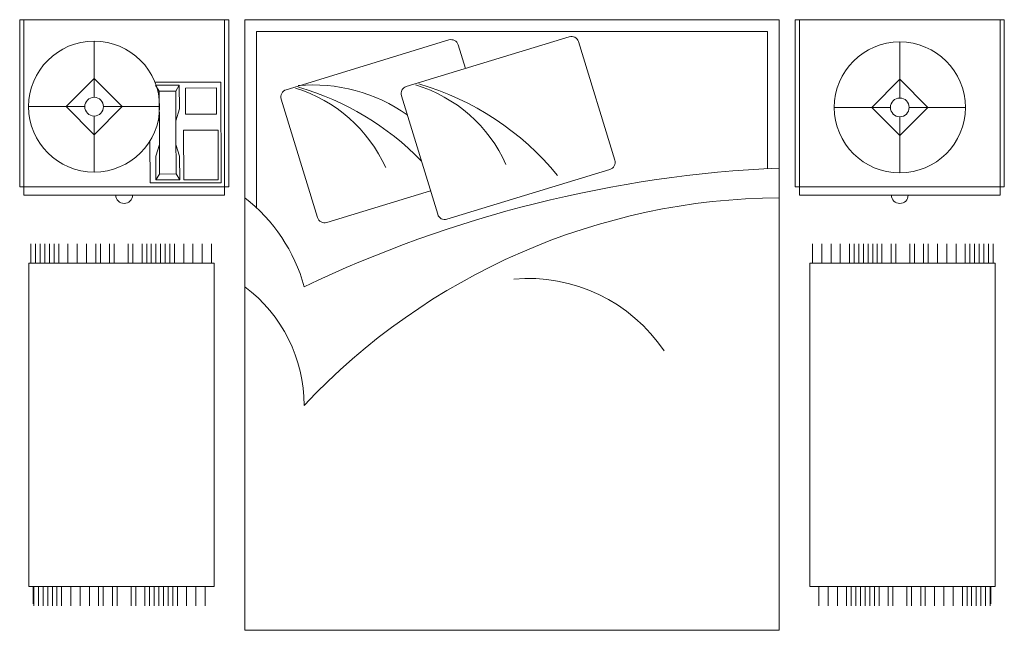
# Model space of a CAD drawing. Units: inches. Extents: x 1994 to 3075, y 3517 to 3950.
# Tile 30 of 58: x 1994.4586 to 1994.5883, y 3553.6956 to 3553.7761. Entities that reach past the tile are written whole.
import ezdxf

# ---------------------------------------------------------------- set-up
doc = ezdxf.new("R2010")
doc.units = ezdxf.units.IN
doc.layers.add('A-FURN-REFR', color=8, linetype='Continuous', lineweight=13)

msp = doc.modelspace()

# ---------------------------------------------------------------- linework, layer by layer
at = {"layer": 'A-FURN-REFR'}
for p, q in [((1994.45855170359, 3553.754079419354), (1994.45855170359, 3553.776112109586)), ((1994.45855170359, 3553.776112109586), (1994.486092566381, 3553.776112109586)), ((1994.459102520846, 3553.752977784842), (1994.459102520846, 3553.776112109586)), ((1994.485541749125, 3553.776112109586), (1994.485541749125, 3553.752977784842)), ((1994.486092566381, 3553.776112109586), (1994.486092566381, 3553.754079419354)), ((1994.488211515722, 3553.776112109586), (1994.488211515722, 3553.752634222582)), ((1994.558645176735, 3553.776112109586), (1994.488211515722, 3553.776112109586)), ((1994.558645176735, 3553.756547203749), (1994.558645176735, 3553.776112109586)), ((1994.560764126075, 3553.776112109586), (1994.560764126075, 3553.754077215864)), ((1994.588307743228, 3553.776112109586), (1994.560764126075, 3553.776112109586)), ((1994.561314998418, 3553.776112109586), (1994.561314998418, 3553.752975471179)), ((1994.587756870884, 3553.752975471179), (1994.587756870884, 3553.776112109586)), ((1994.588307743228, 3553.754077215864), (1994.588307743228, 3553.776112109586)), ((1994.468361056407, 3553.773278802821), (1994.468361056407, 3553.765875817668)), ((1994.515123148426, 3553.773437261622), (1994.493655292272, 3553.766868059838)), ((1994.530971129343, 3553.773869308913), (1994.509503273189, 3553.767300107129)), ((1994.516344913196, 3553.772788026205), (1994.517294663113, 3553.769684286165)), ((1994.532192894112, 3553.773220073496), (1994.536976663113, 3553.757586931427)), ((1994.574535934651, 3553.773181469956), (1994.574535934651, 3553.765777744431)), ((1994.464659560746, 3553.764641987016), (1994.468361056407, 3553.768343480208)), ((1994.468361056407, 3553.768343480208), (1994.472062548366, 3553.764641987016)), ((1994.485054603369, 3553.767890645299), (1994.476376887084, 3553.76785773335)), ((1994.485104968809, 3553.754611060531), (1994.485054603369, 3553.767890645299)), ((1994.574535934651, 3553.768245653762), (1994.570834072506, 3553.764543790383)), ((1994.578237800498, 3553.764543790383), (1994.574535934651, 3553.768245653762)), ((1994.476463412208, 3553.767467479873), (1994.479588020389, 3553.767479330565)), ((1994.476935066108, 3553.766688105432), (1994.476463412208, 3553.767467479873)), ((1994.476935066108, 3553.766688105432), (1994.479122291835, 3553.766696400916)), ((1994.476955804819, 3553.761220041116), (1994.476935066108, 3553.766688105432)), ((1994.479588020389, 3553.767479330565), (1994.479122291835, 3553.766696400916)), ((1994.479143030545, 3553.7612283366), (1994.479122291835, 3553.766696400916)), ((1994.479588020389, 3553.767479330565), (1994.47959987108, 3553.764354722384)), ((1994.493006056854, 3553.765646295068), (1994.497789825855, 3553.750013152999)), ((1994.508854037771, 3553.766078342358), (1994.513637806771, 3553.75044520029)), ((1994.467127225754, 3553.764641987016), (1994.459724238134, 3553.764641987016)), ((1994.468361056407, 3553.760940495056), (1994.464659560746, 3553.764641987016)), ((1994.472062548366, 3553.764641987016), (1994.468361056407, 3553.760940495056)), ((1994.46959488706, 3553.764641987016), (1994.476997870978, 3553.764641987016)), ((1994.47959987108, 3553.764354722384), (1994.479137105199, 3553.762790640691)), ((1994.573301980603, 3553.764543790383), (1994.565898256312, 3553.764543790383)), ((1994.570834072506, 3553.764543790383), (1994.574535934651, 3553.760841928237)), ((1994.574535934651, 3553.760841928237), (1994.578237800498, 3553.764543790383)), ((1994.5757698887, 3553.764543790383), (1994.583173616692, 3553.764543790383)), ((1994.468361056407, 3553.76340815698), (1994.468361056407, 3553.756005173678)), ((1994.476856918961, 3553.763087996861), (1994.476949879473, 3553.762782345206)), ((1994.574535934651, 3553.763309836951), (1994.574535934651, 3553.755906113277)), ((1994.476955804819, 3553.761220041116), (1994.47697654353, 3553.755751976799)), ((1994.479143030545, 3553.7612283366), (1994.479163769256, 3553.755760272284)), ((1994.475710172916, 3553.760104911694), (1994.475731144267, 3553.754575508455)), ((1994.476498964283, 3553.758093655331), (1994.476961730165, 3553.759657737025)), ((1994.479623572464, 3553.758105506023), (1994.479148955892, 3553.759666032509)), ((1994.476510814975, 3553.75496904715), (1994.476498964283, 3553.758093655331)), ((1994.479635423156, 3553.754980897842), (1994.479623572464, 3553.758105506023)), ((1994.536327427695, 3553.756365166657), (1994.514859571541, 3553.749795964872)), ((1994.558645176735, 3553.756547203749), (1994.558645176735, 3553.695576880486)), ((1994.475731144267, 3553.754575508455), (1994.485104968809, 3553.754611060531)), ((1994.47697654353, 3553.755751976799), (1994.476510814975, 3553.75496904715)), ((1994.476510814975, 3553.75496904715), (1994.479635423156, 3553.754980897842)), ((1994.47697654353, 3553.755751976799), (1994.479163769256, 3553.755760272284)), ((1994.479635423156, 3553.754980897842), (1994.479163769256, 3553.755760272284)), ((1994.486092566381, 3553.754079419354), (1994.45855170359, 3553.754079419354)), ((1994.512688056854, 3553.75354894033), (1994.499011590624, 3553.749363917582)), ((1994.560764126075, 3553.754077215864), (1994.588307743228, 3553.754077215864)), ((1994.485541749125, 3553.752977784842), (1994.459102520846, 3553.752977784842)), ((1994.488211515722, 3553.752634222582), (1994.488211515722, 3553.695576880486)), ((1994.561314998418, 3553.752975471179), (1994.587756870884, 3553.752975471179)), ((1994.460028788472, 3553.746531228937, -0.0358017680513295), (1994.460028788472, 3553.743990908382, -0.0358017680513295)), ((1994.460639045881, 3553.746531228937, -0.0358017680513295), (1994.460639045881, 3553.743990908382, -0.0358017680513295)), ((1994.460639045881, 3553.746531228937, -0.0358017680513295), (1994.460639045881, 3553.743990908382, -0.0358017680513295)), ((1994.461249303291, 3553.746531228937, -0.0358017680513295), (1994.461249303291, 3553.743990908382, -0.0358017680513295)), ((1994.461859560701, 3553.746531228937, -0.0358017680513295), (1994.461859560701, 3553.743990908382, -0.0358017680513295)), ((1994.462469818111, 3553.746531228937, -0.0358017680513295), (1994.462469818111, 3553.743990908382, -0.0358017680513295)), ((1994.463080075522, 3553.746531228937, -0.0358017680513295), (1994.463080075522, 3553.743990908382, -0.0358017680513295)), ((1994.463690332931, 3553.746531228937, -0.0358017680513295), (1994.463690332931, 3553.743990908382, -0.0358017680513295)), ((1994.464910847751, 3553.746531228937, -0.0358017680513295), (1994.464910847751, 3553.743990908382, -0.0358017680513295)), ((1994.466131362571, 3553.746531228937, -0.0358017680513295), (1994.466131362571, 3553.743990908382, -0.0358017680513295)), ((1994.467351877391, 3553.746531228937, -0.0358017680513295), (1994.467351877391, 3553.743990908382, -0.0358017680513295)), ((1994.467351877391, 3553.746531228937, -0.0358017680513295), (1994.467351877391, 3553.743990908382, -0.0358017680513295)), ((1994.468572392211, 3553.746531228937, -0.0358017680513295), (1994.468572392211, 3553.743990908382, -0.0358017680513295)), ((1994.469182649621, 3553.746531228937, -0.0358017680513295), (1994.469182649621, 3553.743990908382, -0.0358017680513295)), ((1994.470403164441, 3553.746531228937, -0.0358017680513295), (1994.470403164441, 3553.743990908382, -0.0358017680513295)), ((1994.471013421851, 3553.746531228937, -0.0358017680513295), (1994.471013421851, 3553.743990908382, -0.0358017680513295)), ((1994.472844194081, 3553.746531228937, -0.0358017680513295), (1994.472844194081, 3553.743990908382, -0.0358017680513295)), ((1994.473454451491, 3553.746531228937, -0.0358017680513295), (1994.473454451491, 3553.743990908382, -0.0358017680513295)), ((1994.47467496631, 3553.746531228937, -0.0358017680513295), (1994.47467496631, 3553.743990908382, -0.0358017680513295)), ((1994.475285223721, 3553.746531228937, -0.0358017680513295), (1994.475285223721, 3553.743990908382, -0.0358017680513295)), ((1994.47589548113, 3553.746531228937, -0.0358017680513295), (1994.47589548113, 3553.743990908382, -0.0358017680513295)), ((1994.476505738541, 3553.746531228937, -0.0358017680513295), (1994.476505738541, 3553.743990908382, -0.0358017680513295)), ((1994.47711599595, 3553.746531228937, -0.0358017680513295), (1994.47711599595, 3553.743990908382, -0.0358017680513295)), ((1994.47772625336, 3553.746531228937, -0.0358017680513295), (1994.47772625336, 3553.743990908382, -0.0358017680513295)), ((1994.478336510771, 3553.746531228937, -0.0358017680513295), (1994.478336510771, 3553.743990908382, -0.0358017680513295)), ((1994.47894676818, 3553.746531228937, -0.0358017680513295), (1994.47894676818, 3553.743990908382, -0.0358017680513295)), ((1994.480167283, 3553.746531228937, -0.0358017680513295), (1994.480167283, 3553.743990908382, -0.0358017680513295)), ((1994.48138779782, 3553.746531228937, -0.0358017680513295), (1994.48138779782, 3553.743990908382, -0.0358017680513295)), ((1994.48260831264, 3553.746531228937, -0.0358017680513295), (1994.48260831264, 3553.743990908382, -0.0358017680513295)), ((1994.48382882746, 3553.746531228937, -0.0358017680513295), (1994.48382882746, 3553.743990908382, -0.0358017680513295)), ((1994.563027864996, 3553.746531228937, -0.0358017680513295), (1994.563027864996, 3553.743990908382, -0.0358017680513295)), ((1994.564248379816, 3553.746531228937, -0.0358017680513295), (1994.564248379816, 3553.743990908382, -0.0358017680513295)), ((1994.565468894636, 3553.746531228937, -0.0358017680513295), (1994.565468894636, 3553.743990908382, -0.0358017680513295)), ((1994.566689409456, 3553.746531228937, -0.0358017680513295), (1994.566689409456, 3553.743990908382, -0.0358017680513295)), ((1994.567909924276, 3553.746531228937, -0.0358017680513295), (1994.567909924276, 3553.743990908382, -0.0358017680513295)), ((1994.568520181686, 3553.746531228937, -0.0358017680513295), (1994.568520181686, 3553.743990908382, -0.0358017680513295)), ((1994.569130439096, 3553.746531228937, -0.0358017680513295), (1994.569130439096, 3553.743990908382, -0.0358017680513295)), ((1994.569740696505, 3553.746531228937, -0.0358017680513295), (1994.569740696505, 3553.743990908382, -0.0358017680513295)), ((1994.570350953916, 3553.746531228937, -0.0358017680513295), (1994.570350953916, 3553.743990908382, -0.0358017680513295)), ((1994.570961211326, 3553.746531228937, -0.0358017680513295), (1994.570961211326, 3553.743990908382, -0.0358017680513295)), ((1994.571571468735, 3553.746531228937, -0.0358017680513295), (1994.571571468735, 3553.743990908382, -0.0358017680513295)), ((1994.572181726146, 3553.746531228937, -0.0358017680513295), (1994.572181726146, 3553.743990908382, -0.0358017680513295)), ((1994.573402240965, 3553.746531228937, -0.0358017680513295), (1994.573402240965, 3553.743990908382, -0.0358017680513295)), ((1994.574012498375, 3553.746531228937, -0.0358017680513295), (1994.574012498375, 3553.743990908382, -0.0358017680513295)), ((1994.575843270605, 3553.746531228937, -0.0358017680513295), (1994.575843270605, 3553.743990908382, -0.0358017680513295)), ((1994.576453528015, 3553.746531228937, -0.0358017680513295), (1994.576453528015, 3553.743990908382, -0.0358017680513295)), ((1994.577674042835, 3553.746531228937, -0.0358017680513295), (1994.577674042835, 3553.743990908382, -0.0358017680513295)), ((1994.578284300245, 3553.746531228937, -0.0358017680513295), (1994.578284300245, 3553.743990908382, -0.0358017680513295)), ((1994.579504815065, 3553.746531228937, -0.0358017680513295), (1994.579504815065, 3553.743990908382, -0.0358017680513295)), ((1994.579504815065, 3553.746531228937, -0.0358017680513295), (1994.579504815065, 3553.743990908382, -0.0358017680513295)), ((1994.580725329885, 3553.746531228937, -0.0358017680513295), (1994.580725329885, 3553.743990908382, -0.0358017680513295)), ((1994.581945844705, 3553.746531228937, -0.0358017680513295), (1994.581945844705, 3553.743990908382, -0.0358017680513295)), ((1994.583166359525, 3553.746531228937, -0.0358017680513295), (1994.583166359525, 3553.743990908382, -0.0358017680513295)), ((1994.583776616935, 3553.746531228937, -0.0358017680513295), (1994.583776616935, 3553.743990908382, -0.0358017680513295)), ((1994.584386874345, 3553.746531228937, -0.0358017680513295), (1994.584386874345, 3553.743990908382, -0.0358017680513295)), ((1994.584997131755, 3553.746531228937, -0.0358017680513295), (1994.584997131755, 3553.743990908382, -0.0358017680513295)), ((1994.585607389165, 3553.746531228937, -0.0358017680513295), (1994.585607389165, 3553.743990908382, -0.0358017680513295)), ((1994.586217646575, 3553.746531228937, -0.0358017680513295), (1994.586217646575, 3553.743990908382, -0.0358017680513295)), ((1994.586217646575, 3553.746531228937, -0.0358017680513295), (1994.586217646575, 3553.743990908382, -0.0358017680513295)), ((1994.586827903985, 3553.746531228937, -0.0358017680513295), (1994.586827903985, 3553.743990908382, -0.0358017680513295)), ((1994.459768755177, 3553.743990908382, -0.0358017680513295), (1994.459768755177, 3553.701369855075, -0.0358017680513295)), ((1994.459768755177, 3553.743990908382, -0.0358017680513295), (1994.484179051575, 3553.743990908382, -0.0358017680513295)), ((1994.484179051575, 3553.743990908382, -0.0358017680513295), (1994.484179051575, 3553.701369855075, -0.0358017680513295)), ((1994.587087937279, 3553.743990908382, -0.0358017680513295), (1994.562677640881, 3553.743990908382, -0.0358017680513295)), ((1994.562677640881, 3553.743990908382, -0.0358017680513295), (1994.562677640881, 3553.701369855075, -0.0358017680513295)), ((1994.587087937279, 3553.743990908382, -0.0358017680513295), (1994.587087937279, 3553.701369855075, -0.0358017680513295)), ((1994.459768755177, 3553.701369855075, -0.0358017680513295), (1994.484179051575, 3553.701369855075, -0.0358017680513295)), ((1994.460319196765, 3553.701369855075, -0.0358017680513295), (1994.460319196765, 3553.69905218541, -0.0358017680513295)), ((1994.460319196765, 3553.701369855075, -0.0358017680513295), (1994.460319196765, 3553.69905218541, -0.0358017680513295)), ((1994.460319196765, 3553.701369855075, -0.0358017680513295), (1994.460319196765, 3553.69905218541, -0.0358017680513295)), ((1994.460412957001, 3553.701367703026, -0.0358017680513295), (1994.460412957001, 3553.698827382471, -0.0358017680513295)), ((1994.461023214411, 3553.701367703026, -0.0358017680513295), (1994.461023214411, 3553.698827382471, -0.0358017680513295)), ((1994.461023214411, 3553.701367703026, -0.0358017680513295), (1994.461023214411, 3553.698827382471, -0.0358017680513295)), ((1994.461633471821, 3553.701367703026, -0.0358017680513295), (1994.461633471821, 3553.698827382471, -0.0358017680513295)), ((1994.46224372923, 3553.701367703026, -0.0358017680513295), (1994.46224372923, 3553.698827382471, -0.0358017680513295)), ((1994.462853986641, 3553.701367703026, -0.0358017680513295), (1994.462853986641, 3553.698827382471, -0.0358017680513295)), ((1994.46346424405, 3553.701367703026, -0.0358017680513295), (1994.46346424405, 3553.698827382471, -0.0358017680513295)), ((1994.46407450146, 3553.701367703026, -0.0358017680513295), (1994.46407450146, 3553.698827382471, -0.0358017680513295)), ((1994.46529501628, 3553.701367703026, -0.0358017680513295), (1994.46529501628, 3553.698827382471, -0.0358017680513295)), ((1994.4665155311, 3553.701367703026, -0.0358017680513295), (1994.4665155311, 3553.698827382471, -0.0358017680513295)), ((1994.46773604592, 3553.701367703026, -0.0358017680513295), (1994.46773604592, 3553.698827382471, -0.0358017680513295)), ((1994.46773604592, 3553.701367703026, -0.0358017680513295), (1994.46773604592, 3553.698827382471, -0.0358017680513295)), ((1994.46895656074, 3553.701367703026, -0.0358017680513295), (1994.46895656074, 3553.698827382471, -0.0358017680513295)), ((1994.46956681815, 3553.701367703026, -0.0358017680513295), (1994.46956681815, 3553.698827382471, -0.0358017680513295)), ((1994.47078733297, 3553.701367703026, -0.0358017680513295), (1994.47078733297, 3553.698827382471, -0.0358017680513295)), ((1994.47139759038, 3553.701367703026, -0.0358017680513295), (1994.47139759038, 3553.698827382471, -0.0358017680513295)), ((1994.47322836261, 3553.701367703026, -0.0358017680513295), (1994.47322836261, 3553.698827382471, -0.0358017680513295)), ((1994.47383862002, 3553.701367703026, -0.0358017680513295), (1994.47383862002, 3553.698827382471, -0.0358017680513295)), ((1994.47505913484, 3553.701367703026, -0.0358017680513295), (1994.47505913484, 3553.698827382471, -0.0358017680513295)), ((1994.47566939225, 3553.701367703026, -0.0358017680513295), (1994.47566939225, 3553.698827382471, -0.0358017680513295)), ((1994.47627964966, 3553.701367703026, -0.0358017680513295), (1994.47627964966, 3553.698827382471, -0.0358017680513295)), ((1994.47688990707, 3553.701367703026, -0.0358017680513295), (1994.47688990707, 3553.698827382471, -0.0358017680513295)), ((1994.47750016448, 3553.701367703026, -0.0358017680513295), (1994.47750016448, 3553.698827382471, -0.0358017680513295)), ((1994.47811042189, 3553.701367703026, -0.0358017680513295), (1994.47811042189, 3553.698827382471, -0.0358017680513295)), ((1994.4787206793, 3553.701367703026, -0.0358017680513295), (1994.4787206793, 3553.698827382471, -0.0358017680513295)), ((1994.47933093671, 3553.701367703026, -0.0358017680513295), (1994.47933093671, 3553.698827382471, -0.0358017680513295)), ((1994.48055145153, 3553.701367703026, -0.0358017680513295), (1994.48055145153, 3553.698827382471, -0.0358017680513295)), ((1994.48177196635, 3553.701367703026, -0.0358017680513295), (1994.48177196635, 3553.698827382471, -0.0358017680513295)), ((1994.482992481169, 3553.701367703026, -0.0358017680513295), (1994.482992481169, 3553.698827382471, -0.0358017680513295)), ((1994.587087937279, 3553.701369855075, -0.0358017680513295), (1994.562677640881, 3553.701369855075, -0.0358017680513295)), ((1994.563864211287, 3553.701367703026, -0.0358017680513295), (1994.563864211287, 3553.698827382471, -0.0358017680513295)), ((1994.565084726106, 3553.701367703026, -0.0358017680513295), (1994.565084726106, 3553.698827382471, -0.0358017680513295)), ((1994.566305240926, 3553.701367703026, -0.0358017680513295), (1994.566305240926, 3553.698827382471, -0.0358017680513295)), ((1994.567525755746, 3553.701367703026, -0.0358017680513295), (1994.567525755746, 3553.698827382471, -0.0358017680513295)), ((1994.568136013156, 3553.701367703026, -0.0358017680513295), (1994.568136013156, 3553.698827382471, -0.0358017680513295)), ((1994.568746270567, 3553.701367703026, -0.0358017680513295), (1994.568746270567, 3553.698827382471, -0.0358017680513295)), ((1994.569356527976, 3553.701367703026, -0.0358017680513295), (1994.569356527976, 3553.698827382471, -0.0358017680513295)), ((1994.569966785386, 3553.701367703026, -0.0358017680513295), (1994.569966785386, 3553.698827382471, -0.0358017680513295)), ((1994.570577042796, 3553.701367703026, -0.0358017680513295), (1994.570577042796, 3553.698827382471, -0.0358017680513295)), ((1994.571187300206, 3553.701367703026, -0.0358017680513295), (1994.571187300206, 3553.698827382471, -0.0358017680513295)), ((1994.571797557616, 3553.701367703026, -0.0358017680513295), (1994.571797557616, 3553.698827382471, -0.0358017680513295)), ((1994.573018072436, 3553.701367703026, -0.0358017680513295), (1994.573018072436, 3553.698827382471, -0.0358017680513295)), ((1994.573628329846, 3553.701367703026, -0.0358017680513295), (1994.573628329846, 3553.698827382471, -0.0358017680513295)), ((1994.575459102076, 3553.701367703026, -0.0358017680513295), (1994.575459102076, 3553.698827382471, -0.0358017680513295)), ((1994.576069359486, 3553.701367703026, -0.0358017680513295), (1994.576069359486, 3553.698827382471, -0.0358017680513295)), ((1994.577289874306, 3553.701367703026, -0.0358017680513295), (1994.577289874306, 3553.698827382471, -0.0358017680513295)), ((1994.577900131716, 3553.701367703026, -0.0358017680513295), (1994.577900131716, 3553.698827382471, -0.0358017680513295)), ((1994.579120646536, 3553.701367703026, -0.0358017680513295), (1994.579120646536, 3553.698827382471, -0.0358017680513295)), ((1994.579120646536, 3553.701367703026, -0.0358017680513295), (1994.579120646536, 3553.698827382471, -0.0358017680513295)), ((1994.580341161356, 3553.701367703026, -0.0358017680513295), (1994.580341161356, 3553.698827382471, -0.0358017680513295)), ((1994.581561676176, 3553.701367703026, -0.0358017680513295), (1994.581561676176, 3553.698827382471, -0.0358017680513295)), ((1994.582782190996, 3553.701367703026, -0.0358017680513295), (1994.582782190996, 3553.698827382471, -0.0358017680513295)), ((1994.583392448405, 3553.701367703026, -0.0358017680513295), (1994.583392448405, 3553.698827382471, -0.0358017680513295)), ((1994.584002705815, 3553.701367703026, -0.0358017680513295), (1994.584002705815, 3553.698827382471, -0.0358017680513295)), ((1994.584612963226, 3553.701367703026, -0.0358017680513295), (1994.584612963226, 3553.698827382471, -0.0358017680513295)), ((1994.585223220635, 3553.701367703026, -0.0358017680513295), (1994.585223220635, 3553.698827382471, -0.0358017680513295)), ((1994.585833478046, 3553.701367703026, -0.0358017680513295), (1994.585833478046, 3553.698827382471, -0.0358017680513295)), ((1994.585833478046, 3553.701367703026, -0.0358017680513295), (1994.585833478046, 3553.698827382471, -0.0358017680513295)), ((1994.586443735455, 3553.701367703026, -0.0358017680513295), (1994.586443735455, 3553.698827382471, -0.0358017680513295)), ((1994.586537495691, 3553.701369855075, -0.0358017680513295), (1994.586537495691, 3553.69905218541, -0.0358017680513295)), ((1994.586537495691, 3553.701369855075, -0.0358017680513295), (1994.586537495691, 3553.69905218541, -0.0358017680513295)), ((1994.586537495691, 3553.701369855075, -0.0358017680513295), (1994.586537495691, 3553.69905218541, -0.0358017680513295)), ((1994.488211515722, 3553.695576880486), (1994.558645176735, 3553.695576880486))]:
    msp.add_line(p, q, dxfattribs=at)
msp.add_lwpolyline([(1994.557079984268, 3553.756470188041), (1994.557079984268, 3553.77454691712), (1994.489776708188, 3553.77454691712), (1994.489776708188, 3553.751296470491)], dxfattribs=at)
for points in [[(1994.480409711373, 3553.76709186535), (1994.480422747193, 3553.763654780727), (1994.484484737828, 3553.763670186627), (1994.484471702008, 3553.767107271249)], [(1994.480157343194, 3553.76154463327), (1994.480182229588, 3553.754982971713), (1994.48471291145, 3553.755000155216), (1994.484688025056, 3553.761561816773)]]:
    msp.add_lwpolyline(points, close=True, dxfattribs=at)
for points in [[(1994.488211515722, 3553.752634222582, -0.1622776601683779), (1994.496037478056, 3553.74089527908, -0.1006644078301225), (1994.558645176735, 3553.756547203749, -0.1006644078301225)], [(1994.488211515722, 3553.74089527908, -0.2360679774997873), (1994.496037478056, 3553.72524335441, -0.2052577019546335), (1994.558645176735, 3553.752634222582, -0.2052577019546335)]]:
    msp.add_lwpolyline(points, format="xyb", dxfattribs=at)
for centre, radius in [((1994.468361056407, 3553.764641987016), 0.008636814571209), ((1994.574535934651, 3553.764543790383), 0.0086376783390429), ((1994.468361056407, 3553.764641987016), 0.0012338306530299), ((1994.574535934651, 3553.764543790383), 0.0012339540484347)]:
    msp.add_circle(centre, radius, dxfattribs=at)
for centre, radius, start, end in [((1994.515409413102, 3553.772501761529), 0.0009783189103515, 17.01420295955683, 107.0142029593372), ((1994.531257394019, 3553.772933808819), 0.0009783189103515, 17.01420295955683, 107.0142029593372), ((1994.497181807028, 3553.745989452699), 0.0215272479430675, 54.68510591758633, 95.16051424341522), ((1994.50514269397, 3553.749162519498), 0.0191836131762325, 24.22086799199326, 73.06905818688581), ((1994.500755255058, 3553.732023378153), 0.0371110980284143, 39.40233085362873, 73.71889091943504), ((1994.493941556948, 3553.765932559744), 0.0009783189103515, 107.0142029593372, 197.0142029595568), ((1994.489294713053, 3553.748730472206), 0.0191836131762325, 24.22086799199326, 73.06905818688581), ((1994.484907274141, 3553.731591330862), 0.0371110980284143, 44.27274332327584, 73.71889091943504), ((1994.509789537865, 3553.766364607035), 0.0009783189103515, 107.0142029593372, 197.0142029595568), ((1994.536041163019, 3553.757300666751), 0.0009783189103515, 287.0142029593372, 17.01420295955683), ((1994.472322134986, 3553.752977784842), 0.0011016345116338, 180, 0), ((1994.574535934651, 3553.752975471179), 0.0011017446861024, 180, 0), ((1994.498725325948, 3553.750299417675), 0.0009783189103515, 197.0142029595568, 287.0142029593372), ((1994.514573306865, 3553.750731464966), 0.0009783189103515, 197.0142029595568, 287.0142029593372), ((1994.525588140378, 3553.720453041549), 0.0215272479430652, 33.78007173856782, 95.16051424341522)]:
    msp.add_arc(centre, radius, start, end, dxfattribs=at)

doc.saveas('drawing.dxf')
